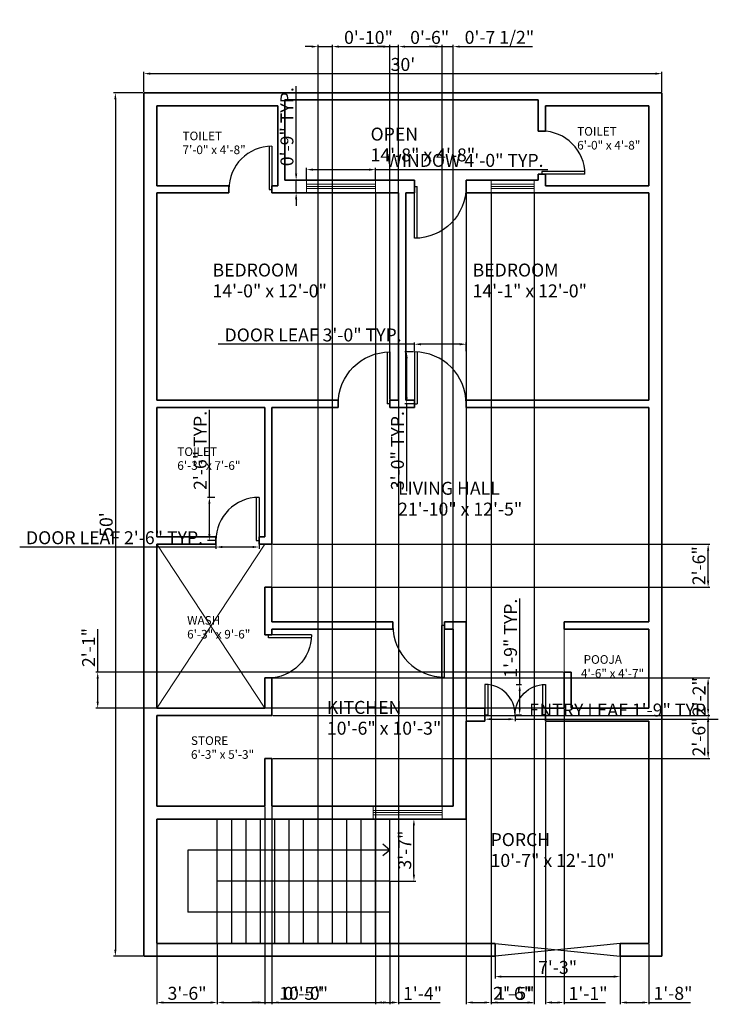
# Model space of a CAD drawing. Units: inches. Extents: x 2391 to 2876, y 1306 to 1990.
import ezdxf

# ---------------------------------------------------------------- set-up
doc = ezdxf.new("R2010")
doc.units = ezdxf.units.IN
for name, color, linetype, lineweight in [('A-ANNO-DIMS', 253, 'Continuous', 18), ('A-AREA-IDEN', 11, 'Continuous', 25), ('A-DOOR', 4, 'Continuous', 25), ('A-FLOR', 11, 'Continuous', 13), ('A-FLOR-STRS', 7, 'Continuous', 25), ('A-GLAZ', 11, 'Continuous', 18), ('A-WALL', 7, 'Continuous', 35), ('A-WALL-OPEN', 11, 'Continuous', 18)]:
    doc.layers.add(name, color=color, linetype=linetype, lineweight=lineweight)
doc.styles.get("Standard").update_dxf_attribs({"font": 'arial.ttf'})
doc.dimstyles.new('ISO-25', dxfattribs={"dimtxt": 9, "dimasz": 4.5, "dimexe": 1.25, "dimexo": 0.625, "dimtad": 1, "dimdec": 0, "dimlunit": 3, "dimtxsty": 'Standard', "dimcen": 2.5, "dimadec": 0, "dimazin": 0, "dimtfac": 1, "dimtdec": 0, "dimtmove": 0, "dimatfit": 3, "dimfxl": 1, "dimarcsym": 0})

# ---------------------------------------------------------------- blocks, each defined once
blk = doc.blocks.new('*D1')
at = {"layer": 'A-ANNO-DIMS', "color": 0, "lineweight": -2, "transparency": 16777216}
for p, q in [((2648.65, 1434.82), (2665.92, 1434.82)), ((2664.67, 1396.12), (2664.67, 1430.32)), ((2648.65, 1391.62), (2665.92, 1391.62))]:
    blk.add_line(p, q, dxfattribs=at)
at = {"layer": 'A-ANNO-DIMS', "color": 0, "transparency": 16777216}
for points in [[(2663.92, 1430.32), (2665.42, 1430.32), (2664.67, 1434.82)], [(2663.92, 1396.12), (2665.42, 1396.12), (2664.67, 1391.62)]]:
    blk.add_solid(points, dxfattribs=at)
at = {"layer": 'Defpoints', "color": 0, "transparency": 16777216}
for p in [(2648.03, 1434.82), (2664.67, 1434.82), (2648.03, 1391.62)]:
    blk.add_point(p, dxfattribs=at)
at = {"layer": 'A-ANNO-DIMS', "color": 0, "transparency": 16777216, "insert": (2659.45, 1413.22), "char_height": 9, "attachment_point": 5, "rotation": 90}
blk.add_mtext('3\'-7"', dxfattribs=at)
blk = doc.blocks.new('*D2')
at = {"layer": 'A-ANNO-DIMS', "color": 0, "lineweight": -2, "transparency": 16777216}
for p, q in [((2721.03, 1347.79), (2721.03, 1324.07)), ((2808.03, 1347.79), (2808.03, 1324.07)), ((2725.53, 1325.32), (2803.53, 1325.32))]:
    blk.add_line(p, q, dxfattribs=at)
at = {"layer": 'A-ANNO-DIMS', "color": 0, "transparency": 16777216}
for points in [[(2725.53, 1326.07), (2725.53, 1324.57), (2721.03, 1325.32)], [(2803.53, 1326.07), (2803.53, 1324.57), (2808.03, 1325.32)]]:
    blk.add_solid(points, dxfattribs=at)
at = {"layer": 'Defpoints', "color": 0, "transparency": 16777216}
for p in [(2721.03, 1348.42), (2808.03, 1348.42), (2808.03, 1325.32)]:
    blk.add_point(p, dxfattribs=at)
at = {"layer": 'A-ANNO-DIMS', "color": 0, "transparency": 16777216, "insert": (2764.53, 1330.54), "char_height": 9, "attachment_point": 5}
blk.add_mtext('7\'-3"', dxfattribs=at)
blk = doc.blocks.new('*D3')
at = {"layer": 'A-ANNO-DIMS', "color": 0, "lineweight": -2, "transparency": 16777216}
for p, q in [((2477.03, 1940.04), (2477.03, 1953.99)), ((2481.53, 1952.74), (2832.53, 1952.74)), ((2837.03, 1940.04), (2837.03, 1953.99))]:
    blk.add_line(p, q, dxfattribs=at)
at = {"layer": 'A-ANNO-DIMS', "color": 0, "transparency": 16777216}
for points in [[(2481.53, 1953.49), (2481.53, 1951.99), (2477.03, 1952.74)], [(2832.53, 1953.49), (2832.53, 1951.99), (2837.03, 1952.74)]]:
    blk.add_solid(points, dxfattribs=at)
at = {"layer": 'Defpoints', "color": 0, "transparency": 16777216}
for p in [(2837.03, 1952.74), (2477.03, 1939.42), (2837.03, 1939.42)]:
    blk.add_point(p, dxfattribs=at)
at = {"layer": 'A-ANNO-DIMS', "color": 0, "transparency": 16777216, "insert": (2657.03, 1957.96), "char_height": 9, "attachment_point": 5}
blk.add_mtext("30'", dxfattribs=at)
blk = doc.blocks.new('*D4')
at = {"layer": 'A-ANNO-DIMS', "color": 0, "lineweight": -2, "transparency": 16777216}
for p, q in [((2476.4, 1939.42), (2455.95, 1939.42)), ((2457.2, 1934.92), (2457.2, 1343.92)), ((2476.4, 1339.42), (2455.95, 1339.42))]:
    blk.add_line(p, q, dxfattribs=at)
at = {"layer": 'A-ANNO-DIMS', "color": 0, "transparency": 16777216}
for points in [[(2456.45, 1934.92), (2457.95, 1934.92), (2457.2, 1939.42)], [(2456.45, 1343.92), (2457.95, 1343.92), (2457.2, 1339.42)]]:
    blk.add_solid(points, dxfattribs=at)
at = {"layer": 'Defpoints', "color": 0, "transparency": 16777216}
for p in [(2477.03, 1939.42), (2457.2, 1339.42), (2477.03, 1339.42)]:
    blk.add_point(p, dxfattribs=at)
at = {"layer": 'A-ANNO-DIMS', "color": 0, "transparency": 16777216, "insert": (2451.98, 1639.42), "char_height": 9, "attachment_point": 5, "rotation": 90}
blk.add_mtext("50'", dxfattribs=at)
blk = doc.blocks.new('DOOR-LEAF-30IN')
for p, q in [((30, 2), (0, 2)), ((0, 2), (0, 0)), ((30, 0), (0, 0))]:
    blk.add_line(p, q)
blk.add_arc((0, 0), 30, 0, 90)
blk = doc.blocks.new('DOOR-LEAF-36IN')
for p, q in [((0, 0), (-2, 0)), ((-2, -36), (-2, 0)), ((0, -36), (0, 0))]:
    blk.add_line(p, q)
blk.add_arc((0, 0), 36, 180, 270)
blk = doc.blocks.new('WIN-48IN')
for p, q in [((0, 0), (48, 0)), ((0, -9), (0, 0)), ((0, -3), (48, -3)), ((0, -4.5), (48, -4.5)), ((0, -6), (48, -6)), ((48, 0), (48, -9)), ((48, -9), (0, -9))]:
    blk.add_line(p, q)
blk = doc.blocks.new('DOOR-LEAF-21IN')
for p, q in [((0, 21), (0, 0)), ((2, 21), (2, 0)), ((0, 0), (2, 0))]:
    blk.add_line(p, q)
blk.add_arc((0, 0), 21, 0, 90)
blk = doc.blocks.new('*D9')
at = {"layer": 'A-ANNO-DIMS', "color": 0, "lineweight": -2, "transparency": 16777216}
for p, q in [((2527.03, 1623.82), (2390.72, 1623.82)), ((2527.03, 1627.69), (2527.03, 1622.57)), ((2552.53, 1623.82), (2531.53, 1623.82)), ((2557.03, 1627.69), (2557.03, 1622.57))]:
    blk.add_line(p, q, dxfattribs=at)
at = {"layer": 'A-ANNO-DIMS', "color": 0, "transparency": 16777216}
for points in [[(2531.53, 1624.57), (2531.53, 1623.07), (2527.03, 1623.82)], [(2552.53, 1624.57), (2552.53, 1623.07), (2557.03, 1623.82)]]:
    blk.add_solid(points, dxfattribs=at)
at = {"layer": 'Defpoints', "color": 0, "transparency": 16777216}
for p in [(2527.03, 1628.32), (2557.03, 1628.32), (2527.03, 1623.82)]:
    blk.add_point(p, dxfattribs=at)
at = {"layer": 'A-ANNO-DIMS', "color": 0, "transparency": 16777216, "insert": (2456.62, 1629.1), "char_height": 9, "attachment_point": 5}
blk.add_mtext('DOOR LEAF 2\'-6" TYP.', dxfattribs=at)
blk = doc.blocks.new('*D10')
at = {"layer": 'A-ANNO-DIMS', "color": 0, "lineweight": -2, "transparency": 16777216}
for p, q in [((2522.53, 1658.32), (2522.53, 1719.08)), ((2526.4, 1658.32), (2521.28, 1658.32)), ((2522.53, 1632.82), (2522.53, 1653.82)), ((2526.4, 1628.32), (2521.28, 1628.32))]:
    blk.add_line(p, q, dxfattribs=at)
at = {"layer": 'A-ANNO-DIMS', "color": 0, "transparency": 16777216}
for points in [[(2521.78, 1653.82), (2523.28, 1653.82), (2522.53, 1658.32)], [(2521.78, 1632.82), (2523.28, 1632.82), (2522.53, 1628.32)]]:
    blk.add_solid(points, dxfattribs=at)
at = {"layer": 'Defpoints', "color": 0, "transparency": 16777216}
for p in [(2522.53, 1658.32), (2527.03, 1658.32), (2527.03, 1628.32)]:
    blk.add_point(p, dxfattribs=at)
at = {"layer": 'A-ANNO-DIMS', "color": 0, "transparency": 16777216, "insert": (2517.31, 1690.95), "char_height": 9, "attachment_point": 5, "rotation": 90}
blk.add_mtext('2\'-6" TYP.', dxfattribs=at)
blk = doc.blocks.new('*D11')
at = {"layer": 'A-ANNO-DIMS', "color": 0, "lineweight": -2, "transparency": 16777216}
for p, q in [((2665.03, 1759.94), (2665.03, 1765.97)), ((2701.03, 1759.94), (2701.03, 1765.97)), ((2665.03, 1764.72), (2528.72, 1764.72)), ((2696.53, 1764.72), (2669.53, 1764.72))]:
    blk.add_line(p, q, dxfattribs=at)
at = {"layer": 'A-ANNO-DIMS', "color": 0, "transparency": 16777216}
for points in [[(2669.53, 1765.47), (2669.53, 1763.97), (2665.03, 1764.72)], [(2696.53, 1765.47), (2696.53, 1763.97), (2701.03, 1764.72)]]:
    blk.add_solid(points, dxfattribs=at)
at = {"layer": 'Defpoints', "color": 0, "transparency": 16777216}
for p in [(2665.03, 1764.72), (2665.03, 1759.32), (2701.03, 1759.32)]:
    blk.add_point(p, dxfattribs=at)
at = {"layer": 'A-ANNO-DIMS', "color": 0, "transparency": 16777216, "insert": (2594.62, 1770), "char_height": 9, "attachment_point": 5}
blk.add_mtext('DOOR LEAF 3\'-0" TYP.', dxfattribs=at)
blk = doc.blocks.new('*D12')
at = {"layer": 'A-ANNO-DIMS', "color": 0, "lineweight": -2, "transparency": 16777216}
for p, q in [((2664.4, 1759.32), (2658.38, 1759.32)), ((2659.63, 1754.82), (2659.63, 1727.82)), ((2664.4, 1723.32), (2658.38, 1723.32)), ((2659.63, 1723.32), (2659.63, 1662.71))]:
    blk.add_line(p, q, dxfattribs=at)
at = {"layer": 'A-ANNO-DIMS', "color": 0, "transparency": 16777216}
for points in [[(2658.88, 1754.82), (2660.38, 1754.82), (2659.63, 1759.32)], [(2658.88, 1727.82), (2660.38, 1727.82), (2659.63, 1723.32)]]:
    blk.add_solid(points, dxfattribs=at)
at = {"layer": 'Defpoints', "color": 0, "transparency": 16777216}
for p in [(2665.03, 1759.32), (2659.63, 1723.32), (2665.03, 1723.32)]:
    blk.add_point(p, dxfattribs=at)
at = {"layer": 'A-ANNO-DIMS', "color": 0, "transparency": 16777216, "insert": (2654.4, 1690.77), "char_height": 9, "attachment_point": 5, "rotation": 90}
blk.add_mtext('3\'-0" TYP.', dxfattribs=at)
blk = doc.blocks.new('*D13')
at = {"layer": 'A-ANNO-DIMS', "color": 0, "lineweight": -2, "transparency": 16777216}
for p, q in [((2714.03, 1506.69), (2714.03, 1502.92)), ((2735.03, 1506.69), (2735.03, 1502.92)), ((2718.53, 1504.17), (2730.53, 1504.17)), ((2735.03, 1504.17), (2876.21, 1504.17))]:
    blk.add_line(p, q, dxfattribs=at)
at = {"layer": 'A-ANNO-DIMS', "color": 0, "transparency": 16777216}
for points in [[(2718.53, 1504.92), (2718.53, 1503.42), (2714.03, 1504.17)], [(2730.53, 1504.92), (2730.53, 1503.42), (2735.03, 1504.17)]]:
    blk.add_solid(points, dxfattribs=at)
at = {"layer": 'Defpoints', "color": 0, "transparency": 16777216}
for p in [(2714.03, 1507.32), (2735.03, 1507.32), (2735.03, 1504.17)]:
    blk.add_point(p, dxfattribs=at)
at = {"layer": 'A-ANNO-DIMS', "color": 0, "transparency": 16777216, "insert": (2807.87, 1509.39), "char_height": 9, "attachment_point": 5}
blk.add_mtext('ENTRY LEAF 1\'-9" TYP.', dxfattribs=at)
blk = doc.blocks.new('*D14')
at = {"layer": 'A-ANNO-DIMS', "color": 0, "lineweight": -2, "transparency": 16777216}
for p, q in [((2738.18, 1528.32), (2738.18, 1588.08)), ((2735.65, 1528.32), (2739.43, 1528.32)), ((2738.18, 1511.82), (2738.18, 1523.82)), ((2735.65, 1507.32), (2739.43, 1507.32))]:
    blk.add_line(p, q, dxfattribs=at)
at = {"layer": 'A-ANNO-DIMS', "color": 0, "transparency": 16777216}
for points in [[(2737.43, 1523.82), (2738.93, 1523.82), (2738.18, 1528.32)], [(2737.43, 1511.82), (2738.93, 1511.82), (2738.18, 1507.32)]]:
    blk.add_solid(points, dxfattribs=at)
at = {"layer": 'Defpoints', "color": 0, "transparency": 16777216}
for p in [(2735.03, 1528.32), (2738.18, 1528.32), (2735.03, 1507.32)]:
    blk.add_point(p, dxfattribs=at)
at = {"layer": 'A-ANNO-DIMS', "color": 0, "transparency": 16777216, "insert": (2732.96, 1560.45), "char_height": 9, "attachment_point": 5, "rotation": 90}
blk.add_mtext('1\'-9" TYP.', dxfattribs=at)
blk = doc.blocks.new('*D15')
at = {"layer": 'A-ANNO-DIMS', "color": 0, "lineweight": -2, "transparency": 16777216}
for p, q in [((2590.03, 1879.44), (2590.03, 1887.27)), ((2594.53, 1886.02), (2633.53, 1886.02)), ((2638.03, 1879.44), (2638.03, 1887.27)), ((2638.03, 1886.02), (2757.67, 1886.02))]:
    blk.add_line(p, q, dxfattribs=at)
at = {"layer": 'A-ANNO-DIMS', "color": 0, "transparency": 16777216}
for points in [[(2594.53, 1886.77), (2594.53, 1885.27), (2590.03, 1886.02)], [(2633.53, 1886.77), (2633.53, 1885.27), (2638.03, 1886.02)]]:
    blk.add_solid(points, dxfattribs=at)
at = {"layer": 'Defpoints', "color": 0, "transparency": 16777216}
for p in [(2638.03, 1886.02), (2590.03, 1878.82), (2638.03, 1878.82)]:
    blk.add_point(p, dxfattribs=at)
at = {"layer": 'A-ANNO-DIMS', "color": 0, "transparency": 16777216, "insert": (2700.1, 1891.3), "char_height": 9, "attachment_point": 5}
blk.add_mtext('WINDOW 4\'-0" TYP.', dxfattribs=at)
blk = doc.blocks.new('*D16')
at = {"layer": 'A-ANNO-DIMS', "color": 0, "lineweight": -2, "transparency": 16777216}
for p, q in [((2582.83, 1883.32), (2582.83, 1943.93)), ((2589.4, 1878.82), (2581.58, 1878.82)), ((2582.83, 1869.82), (2582.83, 1878.82)), ((2589.4, 1869.82), (2581.58, 1869.82)), ((2582.83, 1865.32), (2582.83, 1860.82))]:
    blk.add_line(p, q, dxfattribs=at)
at = {"layer": 'A-ANNO-DIMS', "color": 0, "transparency": 16777216}
for points in [[(2582.08, 1883.32), (2583.58, 1883.32), (2582.83, 1878.82)], [(2582.08, 1865.32), (2583.58, 1865.32), (2582.83, 1869.82)]]:
    blk.add_solid(points, dxfattribs=at)
at = {"layer": 'Defpoints', "color": 0, "transparency": 16777216}
for p in [(2582.83, 1878.82), (2590.03, 1878.82), (2590.03, 1869.82)]:
    blk.add_point(p, dxfattribs=at)
at = {"layer": 'A-ANNO-DIMS', "color": 0, "transparency": 16777216, "insert": (2577.61, 1915.87), "char_height": 9, "attachment_point": 5, "rotation": 90}
blk.add_mtext('0\'-9" TYP.', dxfattribs=at)
blk = doc.blocks.new('*D17')
at = {"layer": 'A-ANNO-DIMS', "color": 0, "lineweight": -2, "transparency": 16777216}
for p, q in [((2444.93, 1536.82), (2444.93, 1566.65)), ((2768.4, 1536.82), (2443.68, 1536.82)), ((2444.93, 1516.32), (2444.93, 1532.32)), ((2768.4, 1511.82), (2443.68, 1511.82))]:
    blk.add_line(p, q, dxfattribs=at)
at = {"layer": 'A-ANNO-DIMS', "color": 0, "transparency": 16777216}
for points in [[(2444.18, 1532.32), (2445.68, 1532.32), (2444.93, 1536.82)], [(2444.18, 1516.32), (2445.68, 1516.32), (2444.93, 1511.82)]]:
    blk.add_solid(points, dxfattribs=at)
at = {"layer": 'Defpoints', "color": 0, "transparency": 16777216}
for p in [(2444.93, 1536.82), (2769.03, 1536.82), (2769.03, 1511.82)]:
    blk.add_point(p, dxfattribs=at)
at = {"layer": 'A-ANNO-DIMS', "color": 0, "transparency": 16777216, "insert": (2439.78, 1553.98), "char_height": 9, "attachment_point": 5, "rotation": 90}
blk.add_mtext('2\'-1"', dxfattribs=at)
blk = doc.blocks.new('*D18')
at = {"layer": 'A-ANNO-DIMS', "color": 0, "lineweight": -2, "transparency": 16777216}
for p, q in [((2528.03, 1347.79), (2528.03, 1306.07)), ((2648.03, 1347.79), (2648.03, 1306.07)), ((2532.53, 1307.32), (2643.53, 1307.32))]:
    blk.add_line(p, q, dxfattribs=at)
at = {"layer": 'A-ANNO-DIMS', "color": 0, "transparency": 16777216}
for points in [[(2532.53, 1308.07), (2532.53, 1306.57), (2528.03, 1307.32)], [(2643.53, 1308.07), (2643.53, 1306.57), (2648.03, 1307.32)]]:
    blk.add_solid(points, dxfattribs=at)
at = {"layer": 'Defpoints', "color": 0, "transparency": 16777216}
for p in [(2528.03, 1348.42), (2648.03, 1348.42), (2648.03, 1307.32)]:
    blk.add_point(p, dxfattribs=at)
at = {"layer": 'A-ANNO-DIMS', "color": 0, "transparency": 16777216, "insert": (2588.03, 1312.54), "char_height": 9, "attachment_point": 5}
blk.add_mtext('10\'-0"', dxfattribs=at)
blk = doc.blocks.new('*D19')
at = {"layer": 'A-ANNO-DIMS', "color": 0, "lineweight": -2, "transparency": 16777216}
for p, q in [((2486.03, 1347.79), (2486.03, 1306.07)), ((2528.03, 1347.79), (2528.03, 1306.07)), ((2490.53, 1307.32), (2523.53, 1307.32))]:
    blk.add_line(p, q, dxfattribs=at)
at = {"layer": 'A-ANNO-DIMS', "color": 0, "transparency": 16777216}
for points in [[(2490.53, 1308.07), (2490.53, 1306.57), (2486.03, 1307.32)], [(2523.53, 1308.07), (2523.53, 1306.57), (2528.03, 1307.32)]]:
    blk.add_solid(points, dxfattribs=at)
at = {"layer": 'Defpoints', "color": 0, "transparency": 16777216}
for p in [(2486.03, 1348.42), (2528.03, 1348.42), (2528.03, 1307.32)]:
    blk.add_point(p, dxfattribs=at)
at = {"layer": 'A-ANNO-DIMS', "color": 0, "transparency": 16777216, "insert": (2507.03, 1312.54), "char_height": 9, "attachment_point": 5}
blk.add_mtext('3\'-6"', dxfattribs=at)
blk = doc.blocks.new('*D20')
at = {"layer": 'A-ANNO-DIMS', "color": 0, "lineweight": -2, "transparency": 16777216}
for p, q in [((2808.03, 1347.79), (2808.03, 1306.07)), ((2828.03, 1347.79), (2828.03, 1306.07)), ((2812.53, 1307.32), (2823.53, 1307.32)), ((2828.03, 1307.32), (2856.86, 1307.32))]:
    blk.add_line(p, q, dxfattribs=at)
at = {"layer": 'A-ANNO-DIMS', "color": 0, "transparency": 16777216}
for points in [[(2812.53, 1308.07), (2812.53, 1306.57), (2808.03, 1307.32)], [(2823.53, 1308.07), (2823.53, 1306.57), (2828.03, 1307.32)]]:
    blk.add_solid(points, dxfattribs=at)
at = {"layer": 'Defpoints', "color": 0, "transparency": 16777216}
for p in [(2808.03, 1348.42), (2828.03, 1348.42), (2828.03, 1307.32)]:
    blk.add_point(p, dxfattribs=at)
at = {"layer": 'A-ANNO-DIMS', "color": 0, "transparency": 16777216, "insert": (2844.69, 1312.54), "char_height": 9, "attachment_point": 5}
blk.add_mtext('1\'-8"', dxfattribs=at)
blk = doc.blocks.new('*D21')
at = {"layer": 'A-ANNO-DIMS', "color": 0, "lineweight": -2, "transparency": 16777216}
for p, q in [((2566.65, 1506.82), (2870.38, 1506.82)), ((2869.13, 1481.32), (2869.13, 1502.32)), ((2566.65, 1476.82), (2870.38, 1476.82))]:
    blk.add_line(p, q, dxfattribs=at)
at = {"layer": 'A-ANNO-DIMS', "color": 0, "transparency": 16777216}
for points in [[(2868.38, 1502.32), (2869.88, 1502.32), (2869.13, 1506.82)], [(2868.38, 1481.32), (2869.88, 1481.32), (2869.13, 1476.82)]]:
    blk.add_solid(points, dxfattribs=at)
at = {"layer": 'Defpoints', "color": 0, "transparency": 16777216}
for p in [(2566.03, 1506.82), (2869.13, 1506.82), (2566.03, 1476.82)]:
    blk.add_point(p, dxfattribs=at)
at = {"layer": 'A-ANNO-DIMS', "color": 0, "transparency": 16777216, "insert": (2863.91, 1491.82), "char_height": 9, "attachment_point": 5, "rotation": 90}
blk.add_mtext('2\'-6"', dxfattribs=at)
blk = doc.blocks.new('*D22')
at = {"layer": 'A-ANNO-DIMS', "color": 0, "lineweight": -2, "transparency": 16777216}
for p, q in [((2566.65, 1625.82), (2870.38, 1625.82)), ((2869.13, 1600.32), (2869.13, 1621.32)), ((2566.65, 1595.82), (2870.38, 1595.82))]:
    blk.add_line(p, q, dxfattribs=at)
at = {"layer": 'A-ANNO-DIMS', "color": 0, "transparency": 16777216}
for points in [[(2868.38, 1621.32), (2869.88, 1621.32), (2869.13, 1625.82)], [(2868.38, 1600.32), (2869.88, 1600.32), (2869.13, 1595.82)]]:
    blk.add_solid(points, dxfattribs=at)
at = {"layer": 'Defpoints', "color": 0, "transparency": 16777216}
for p in [(2566.03, 1625.82), (2869.13, 1625.82), (2566.03, 1595.82)]:
    blk.add_point(p, dxfattribs=at)
at = {"layer": 'A-ANNO-DIMS', "color": 0, "transparency": 16777216, "insert": (2863.91, 1610.82), "char_height": 9, "attachment_point": 5, "rotation": 90}
blk.add_mtext('2\'-6"', dxfattribs=at)
blk = doc.blocks.new('*D23')
at = {"layer": 'A-ANNO-DIMS', "color": 0, "lineweight": -2, "transparency": 16777216}
for p, q in [((2566.65, 1532.82), (2870.38, 1532.82)), ((2869.13, 1511.32), (2869.13, 1528.32)), ((2566.65, 1506.82), (2870.38, 1506.82))]:
    blk.add_line(p, q, dxfattribs=at)
at = {"layer": 'A-ANNO-DIMS', "color": 0, "transparency": 16777216}
for points in [[(2868.38, 1528.32), (2869.88, 1528.32), (2869.13, 1532.82)], [(2868.38, 1511.32), (2869.88, 1511.32), (2869.13, 1506.82)]]:
    blk.add_solid(points, dxfattribs=at)
at = {"layer": 'Defpoints', "color": 0, "transparency": 16777216}
for p in [(2566.03, 1532.82), (2869.13, 1532.82), (2566.03, 1506.82)]:
    blk.add_point(p, dxfattribs=at)
at = {"layer": 'A-ANNO-DIMS', "color": 0, "transparency": 16777216, "insert": (2863.98, 1519.82), "char_height": 9, "attachment_point": 5, "rotation": 90}
blk.add_mtext('2\'-2"', dxfattribs=at)
blk = doc.blocks.new('*D24')
at = {"layer": 'A-ANNO-DIMS', "color": 0, "lineweight": -2, "transparency": 16777216}
for p, q in [((2638.03, 1869.19), (2638.03, 1306.07)), ((2654.03, 1869.19), (2654.03, 1306.07)), ((2642.53, 1307.32), (2649.53, 1307.32)), ((2654.03, 1307.32), (2682.86, 1307.32))]:
    blk.add_line(p, q, dxfattribs=at)
at = {"layer": 'A-ANNO-DIMS', "color": 0, "transparency": 16777216}
for points in [[(2642.53, 1308.07), (2642.53, 1306.57), (2638.03, 1307.32)], [(2649.53, 1308.07), (2649.53, 1306.57), (2654.03, 1307.32)]]:
    blk.add_solid(points, dxfattribs=at)
at = {"layer": 'Defpoints', "color": 0, "transparency": 16777216}
for p in [(2638.03, 1869.82), (2654.03, 1869.82), (2654.03, 1307.32)]:
    blk.add_point(p, dxfattribs=at)
at = {"layer": 'A-ANNO-DIMS', "color": 0, "transparency": 16777216, "insert": (2670.69, 1312.46), "char_height": 9, "attachment_point": 5}
blk.add_mtext('1\'-4"', dxfattribs=at)
blk = doc.blocks.new('*D25')
at = {"layer": 'A-ANNO-DIMS', "color": 0, "lineweight": -2, "transparency": 16777216}
for p, q in [((2701.03, 1869.19), (2701.03, 1306.07)), ((2718.25, 1869.19), (2718.25, 1306.07)), ((2705.53, 1307.32), (2713.75, 1307.32)), ((2718.25, 1307.32), (2747.07, 1307.32))]:
    blk.add_line(p, q, dxfattribs=at)
at = {"layer": 'A-ANNO-DIMS', "color": 0, "transparency": 16777216}
for points in [[(2705.53, 1308.07), (2705.53, 1306.57), (2701.03, 1307.32)], [(2713.75, 1308.07), (2713.75, 1306.57), (2718.25, 1307.32)]]:
    blk.add_solid(points, dxfattribs=at)
at = {"layer": 'Defpoints', "color": 0, "transparency": 16777216}
for p in [(2701.03, 1869.82), (2718.25, 1869.82), (2718.25, 1307.32)]:
    blk.add_point(p, dxfattribs=at)
at = {"layer": 'A-ANNO-DIMS', "color": 0, "transparency": 16777216, "insert": (2734.91, 1312.54), "char_height": 9, "attachment_point": 5}
blk.add_mtext('1\'-5"', dxfattribs=at)
blk = doc.blocks.new('*D26')
at = {"layer": 'A-ANNO-DIMS', "color": 0, "lineweight": -2, "transparency": 16777216}
for p, q in [((2718.25, 1869.19), (2718.25, 1306.07)), ((2748.25, 1869.19), (2748.25, 1306.07)), ((2722.75, 1307.32), (2743.75, 1307.32))]:
    blk.add_line(p, q, dxfattribs=at)
at = {"layer": 'A-ANNO-DIMS', "color": 0, "transparency": 16777216}
for points in [[(2722.75, 1308.07), (2722.75, 1306.57), (2718.25, 1307.32)], [(2743.75, 1308.07), (2743.75, 1306.57), (2748.25, 1307.32)]]:
    blk.add_solid(points, dxfattribs=at)
at = {"layer": 'Defpoints', "color": 0, "transparency": 16777216}
for p in [(2718.25, 1869.82), (2748.25, 1869.82), (2748.25, 1307.32)]:
    blk.add_point(p, dxfattribs=at)
at = {"layer": 'A-ANNO-DIMS', "color": 0, "transparency": 16777216, "insert": (2733.25, 1312.54), "char_height": 9, "attachment_point": 5}
blk.add_mtext('2\'-6"', dxfattribs=at)
blk = doc.blocks.new('*D27')
at = {"layer": 'A-ANNO-DIMS', "color": 0, "lineweight": -2, "transparency": 16777216}
for p, q in [((2643.53, 1971.52), (2639.03, 1971.52)), ((2648.03, 1726.44), (2648.03, 1972.77)), ((2648.03, 1971.52), (2654.03, 1971.52)), ((2654.03, 1726.44), (2654.03, 1972.77)), ((2658.53, 1971.52), (2688.2, 1971.52))]:
    blk.add_line(p, q, dxfattribs=at)
at = {"layer": 'A-ANNO-DIMS', "color": 0, "transparency": 16777216}
for points in [[(2643.53, 1972.27), (2643.53, 1970.77), (2648.03, 1971.52)], [(2658.53, 1972.27), (2658.53, 1970.77), (2654.03, 1971.52)]]:
    blk.add_solid(points, dxfattribs=at)
at = {"layer": 'Defpoints', "color": 0, "transparency": 16777216}
for p in [(2654.03, 1971.52), (2648.03, 1725.82), (2654.03, 1725.82)]:
    blk.add_point(p, dxfattribs=at)
at = {"layer": 'A-ANNO-DIMS', "color": 0, "transparency": 16777216, "insert": (2675.62, 1976.74), "char_height": 9, "attachment_point": 5}
blk.add_mtext('0\'-6"', dxfattribs=at)
blk = doc.blocks.new('*D28')
at = {"layer": 'A-ANNO-DIMS', "color": 0, "lineweight": -2, "transparency": 16777216}
for p, q in [((2769.03, 1511.19), (2769.03, 1306.07)), ((2756.03, 1502.19), (2756.03, 1306.07)), ((2760.53, 1307.32), (2764.53, 1307.32)), ((2769.03, 1307.32), (2797.86, 1307.32))]:
    blk.add_line(p, q, dxfattribs=at)
at = {"layer": 'A-ANNO-DIMS', "color": 0, "transparency": 16777216}
for points in [[(2760.53, 1308.07), (2760.53, 1306.57), (2756.03, 1307.32)], [(2764.53, 1308.07), (2764.53, 1306.57), (2769.03, 1307.32)]]:
    blk.add_solid(points, dxfattribs=at)
at = {"layer": 'Defpoints', "color": 0, "transparency": 16777216}
for p in [(2769.03, 1511.82), (2756.03, 1502.82), (2769.03, 1307.32)]:
    blk.add_point(p, dxfattribs=at)
at = {"layer": 'A-ANNO-DIMS', "color": 0, "transparency": 16777216, "insert": (2785.69, 1312.46), "char_height": 9, "attachment_point": 5}
blk.add_mtext('1\'-1"', dxfattribs=at)
blk = doc.blocks.new('*D29')
at = {"layer": 'A-ANNO-DIMS', "color": 0, "lineweight": -2, "transparency": 16777216}
for p, q in [((2679.81, 1971.52), (2675.31, 1971.52)), ((2684.31, 1444.44), (2684.31, 1972.77)), ((2684.31, 1971.52), (2692.03, 1971.52)), ((2692.03, 1444.44), (2692.03, 1972.77)), ((2696.53, 1971.52), (2747.17, 1971.52))]:
    blk.add_line(p, q, dxfattribs=at)
at = {"layer": 'A-ANNO-DIMS', "color": 0, "transparency": 16777216}
for points in [[(2679.81, 1972.27), (2679.81, 1970.77), (2684.31, 1971.52)], [(2696.53, 1972.27), (2696.53, 1970.77), (2692.03, 1971.52)]]:
    blk.add_solid(points, dxfattribs=at)
at = {"layer": 'Defpoints', "color": 0, "transparency": 16777216}
for p in [(2692.03, 1971.52), (2684.31, 1443.82), (2692.03, 1443.82)]:
    blk.add_point(p, dxfattribs=at)
at = {"layer": 'A-ANNO-DIMS', "color": 0, "transparency": 16777216, "insert": (2724.1, 1976.8), "char_height": 9, "attachment_point": 5}
blk.add_mtext('0\'-7 1/2"', dxfattribs=at)
blk = doc.blocks.new('*D30')
at = {"layer": 'A-ANNO-DIMS', "color": 0, "lineweight": -2, "transparency": 16777216}
for p, q in [((2561.03, 1443.19), (2561.03, 1306.07)), ((2566.03, 1443.19), (2566.03, 1306.07)), ((2556.53, 1307.32), (2552.03, 1307.32)), ((2561.03, 1307.32), (2566.03, 1307.32)), ((2570.53, 1307.32), (2600.2, 1307.32))]:
    blk.add_line(p, q, dxfattribs=at)
at = {"layer": 'A-ANNO-DIMS', "color": 0, "transparency": 16777216}
for points in [[(2556.53, 1308.07), (2556.53, 1306.57), (2561.03, 1307.32)], [(2570.53, 1308.07), (2570.53, 1306.57), (2566.03, 1307.32)]]:
    blk.add_solid(points, dxfattribs=at)
at = {"layer": 'Defpoints', "color": 0, "transparency": 16777216}
for p in [(2561.03, 1443.82), (2566.03, 1443.82), (2566.03, 1307.32)]:
    blk.add_point(p, dxfattribs=at)
at = {"layer": 'A-ANNO-DIMS', "color": 0, "transparency": 16777216, "insert": (2587.62, 1312.54), "char_height": 9, "attachment_point": 5}
blk.add_mtext('0\'-5"', dxfattribs=at)
blk = doc.blocks.new('*D31')
at = {"layer": 'A-ANNO-DIMS', "color": 0, "lineweight": -2, "transparency": 16777216}
for p, q in [((2593.53, 1971.52), (2589.03, 1971.52)), ((2598.03, 1435.44), (2598.03, 1972.77)), ((2598.03, 1971.52), (2608.03, 1971.52)), ((2608.03, 1435.44), (2608.03, 1972.77)), ((2612.53, 1971.52), (2649.19, 1971.52))]:
    blk.add_line(p, q, dxfattribs=at)
at = {"layer": 'A-ANNO-DIMS', "color": 0, "transparency": 16777216}
for points in [[(2593.53, 1972.27), (2593.53, 1970.77), (2598.03, 1971.52)], [(2612.53, 1972.27), (2612.53, 1970.77), (2608.03, 1971.52)]]:
    blk.add_solid(points, dxfattribs=at)
at = {"layer": 'Defpoints', "color": 0, "transparency": 16777216}
for p in [(2608.03, 1971.52), (2598.03, 1434.82), (2608.03, 1434.82)]:
    blk.add_point(p, dxfattribs=at)
at = {"layer": 'A-ANNO-DIMS', "color": 0, "transparency": 16777216, "insert": (2633.11, 1976.74), "char_height": 9, "attachment_point": 5}
blk.add_mtext('0\'-10"', dxfattribs=at)

msp = doc.modelspace()

# ---------------------------------------------------------------- linework, layer by layer
at = {"layer": 'A-DOOR'}
for p, q in [((2753.53, 1882.82), (2751.53, 1882.82)), ((2721.03, 1348.42), (2808.03, 1339.42)), ((2808.03, 1348.42), (2721.03, 1339.42))]:
    msp.add_line(p, q, dxfattribs=at)
at = {"layer": 'A-FLOR'}
for p, q in [((2486.03, 1625.82), (2561.03, 1511.82)), ((2561.03, 1625.82), (2486.03, 1511.82))]:
    msp.add_line(p, q, dxfattribs=at)
at = {"layer": 'A-FLOR-STRS'}
for p, q in [((2528.03, 1348.42), (2528.03, 1434.82)), ((2538.03, 1348.42), (2538.03, 1434.82)), ((2548.03, 1348.42), (2548.03, 1434.82)), ((2558.03, 1348.42), (2558.03, 1434.82)), ((2568.03, 1348.42), (2568.03, 1434.82)), ((2578.03, 1348.42), (2578.03, 1434.82)), ((2588.03, 1348.42), (2588.03, 1434.82)), ((2598.03, 1348.42), (2598.03, 1434.82)), ((2608.03, 1348.42), (2608.03, 1434.82)), ((2618.03, 1348.42), (2618.03, 1434.82)), ((2628.03, 1348.42), (2628.03, 1434.82)), ((2638.03, 1348.42), (2638.03, 1434.82)), ((2648.03, 1348.42), (2648.03, 1434.82)), ((2648.03, 1391.62), (2648.03, 1434.82)), ((2648.03, 1413.22), (2643, 1417.29)), ((2648.03, 1413.22), (2507.48, 1413.22)), ((2507.48, 1413.22), (2507.48, 1370.02)), ((2648.03, 1413.22), (2643, 1409.15)), ((2648.03, 1391.62), (2528.03, 1391.62)), ((2648.03, 1391.62), (2648.03, 1348.42)), ((2648.03, 1370.02), (2507.48, 1370.02))]:
    msp.add_line(p, q, dxfattribs=at)
at = {"layer": 'A-GLAZ'}
for p, q in [((2718.25, 1878.82), (2718.25, 1869.82)), ((2718.25, 1878.82), (2748.25, 1878.82)), ((2748.25, 1875.82), (2718.25, 1875.82)), ((2748.25, 1878.82), (2748.25, 1869.82)), ((2748.25, 1874.32), (2718.25, 1874.32)), ((2748.25, 1872.82), (2718.25, 1872.82)), ((2718.25, 1869.82), (2748.25, 1869.82))]:
    msp.add_line(p, q, dxfattribs=at)
at = {"layer": 'A-WALL'}
for p, q in [((2477.03, 1939.42), (2837.03, 1939.42)), ((2477.03, 1339.42), (2477.03, 1939.42)), ((2837.03, 1939.42), (2837.03, 1339.42)), ((2486.03, 1930.42), (2570.03, 1930.42)), ((2486.03, 1874.82), (2486.03, 1930.42)), ((2570.03, 1874.82), (2570.03, 1930.42)), ((2575.03, 1878.82), (2575.03, 1934.42)), ((2575.03, 1934.42), (2751.03, 1934.42)), ((2751.03, 1934.42), (2751.03, 1912.82)), ((2756.03, 1930.42), (2756.03, 1912.82)), ((2756.03, 1930.42), (2828.03, 1930.42)), ((2828.03, 1930.42), (2828.03, 1874.82)), ((2751.03, 1912.82), (2756.03, 1912.82)), ((2751.03, 1882.82), (2756.03, 1882.82)), ((2751.03, 1882.82), (2751.03, 1878.82)), ((2756.03, 1882.82), (2756.03, 1874.82)), ((2486.03, 1874.82), (2536.03, 1874.82)), ((2536.03, 1869.82), (2536.03, 1874.82)), ((2566.03, 1869.82), (2566.03, 1874.82)), ((2566.03, 1874.82), (2570.03, 1874.82)), ((2575.03, 1878.82), (2665.03, 1878.82)), ((2665.03, 1869.82), (2665.03, 1878.82)), ((2701.03, 1869.82), (2701.03, 1878.82)), ((2701.03, 1878.82), (2751.03, 1878.82)), ((2756.03, 1874.82), (2828.03, 1874.82)), ((2486.03, 1869.82), (2536.03, 1869.82)), ((2486.03, 1725.82), (2486.03, 1869.82)), ((2566.03, 1869.82), (2654.03, 1869.82)), ((2654.03, 1725.82), (2654.03, 1869.82)), ((2659.03, 1725.82), (2659.03, 1869.82)), ((2659.03, 1869.82), (2665.03, 1869.82)), ((2701.03, 1869.82), (2828.03, 1869.82)), ((2828.03, 1869.82), (2828.03, 1725.82)), ((2486.03, 1725.82), (2612.03, 1725.82)), ((2612.03, 1720.82), (2612.03, 1725.82)), ((2648.03, 1720.82), (2648.03, 1725.82)), ((2648.03, 1725.82), (2654.03, 1725.82)), ((2659.03, 1725.82), (2665.03, 1725.82)), ((2665.03, 1720.82), (2665.03, 1725.82)), ((2665.03, 1720.82), (2665.03, 1725.82)), ((2701.03, 1720.82), (2701.03, 1725.82)), ((2701.03, 1725.82), (2828.03, 1725.82)), ((2701.03, 1720.82), (2701.03, 1725.82)), ((2486.03, 1720.82), (2561.03, 1720.82)), ((2486.03, 1630.82), (2486.03, 1720.82)), ((2561.03, 1630.82), (2561.03, 1720.82)), ((2566.03, 1720.82), (2612.03, 1720.82)), ((2566.03, 1625.82), (2566.03, 1720.82)), ((2648.03, 1720.82), (2665.03, 1720.82)), ((2701.03, 1720.82), (2828.03, 1720.82)), ((2828.03, 1720.82), (2828.03, 1571.82)), ((2486.03, 1630.82), (2527.03, 1630.82)), ((2527.03, 1625.82), (2527.03, 1630.82)), ((2557.03, 1625.82), (2557.03, 1630.82)), ((2557.03, 1630.82), (2561.03, 1630.82)), ((2486.03, 1625.82), (2527.03, 1625.82)), ((2486.03, 1511.82), (2486.03, 1625.82)), ((2557.03, 1625.82), (2566.03, 1625.82)), ((2561.03, 1562.82), (2561.03, 1595.82)), ((2561.03, 1595.82), (2566.03, 1595.82)), ((2566.03, 1571.82), (2566.03, 1595.82)), ((2566.03, 1571.82), (2650.03, 1571.82)), ((2566.03, 1566.82), (2650.03, 1566.82)), ((2566.03, 1562.82), (2566.03, 1566.82)), ((2650.03, 1566.82), (2650.03, 1571.82)), ((2686.03, 1566.82), (2686.03, 1571.82)), ((2686.03, 1571.82), (2701.03, 1571.82)), ((2686.03, 1566.82), (2692.03, 1566.82)), ((2692.03, 1443.82), (2692.03, 1566.82)), ((2701.03, 1511.82), (2701.03, 1571.82)), ((2769.03, 1571.82), (2769.03, 1566.82)), ((2769.03, 1571.82), (2828.03, 1571.82)), ((2769.03, 1566.82), (2828.03, 1566.82)), ((2828.03, 1566.82), (2828.03, 1511.82)), ((2561.03, 1562.82), (2566.03, 1562.82)), ((2561.03, 1532.82), (2566.03, 1532.82)), ((2561.03, 1511.82), (2561.03, 1532.82)), ((2566.03, 1506.82), (2566.03, 1532.82)), ((2769.03, 1536.82), (2774.03, 1536.82)), ((2769.03, 1536.82), (2769.03, 1511.82)), ((2774.03, 1536.82), (2774.03, 1511.82)), ((2486.03, 1511.82), (2561.03, 1511.82)), ((2486.03, 1506.82), (2566.03, 1506.82)), ((2486.03, 1443.82), (2486.03, 1506.82)), ((2701.03, 1511.82), (2714.03, 1511.82)), ((2701.03, 1511.82), (2714.03, 1511.82)), ((2714.03, 1511.82), (2714.03, 1502.82)), ((2756.03, 1511.82), (2756.03, 1502.82)), ((2756.03, 1511.82), (2769.03, 1511.82)), ((2756.03, 1511.82), (2769.03, 1511.82)), ((2774.03, 1511.82), (2828.03, 1511.82)), ((2701.03, 1434.82), (2701.03, 1502.82)), ((2701.03, 1502.82), (2714.03, 1502.82)), ((2756.03, 1502.82), (2828.03, 1502.82)), ((2828.03, 1502.82), (2828.03, 1348.42)), ((2561.03, 1443.82), (2561.03, 1476.82)), ((2561.03, 1476.82), (2566.03, 1476.82)), ((2566.03, 1443.82), (2566.03, 1476.82)), ((2486.03, 1443.82), (2561.03, 1443.82)), ((2566.03, 1443.82), (2692.03, 1443.82)), ((2486.03, 1348.42), (2486.03, 1434.82)), ((2486.03, 1434.82), (2701.03, 1434.82)), ((2721.03, 1348.42), (2486.03, 1348.42)), ((2721.03, 1339.42), (2721.03, 1348.42)), ((2828.03, 1348.42), (2808.03, 1348.42)), ((2808.03, 1348.42), (2808.03, 1339.42)), ((2721.03, 1339.42), (2477.03, 1339.42)), ((2837.03, 1339.42), (2808.03, 1339.42))]:
    msp.add_line(p, q, dxfattribs=at)
at = {"layer": 'A-WALL-OPEN'}
for p, q in [((2566.03, 1625.82), (2566.03, 1595.82)), ((2769.03, 1566.82), (2769.03, 1536.82))]:
    msp.add_line(p, q, dxfattribs=at)

# ---------------------------------------------------------------- block references
at = {"layer": 'A-DOOR'}
for name, p in [('DOOR-LEAF-30IN', (2753.53, 1882.82)), ('DOOR-LEAF-36IN', (2686.03, 1569.32)), ('DOOR-LEAF-21IN', (2714.03, 1507.32))]:
    msp.add_blockref(name, p, dxfattribs=at)
for name, p, rotation in [('DOOR-LEAF-30IN', (2566.03, 1872.32), 90.00000000000003), ('DOOR-LEAF-36IN', (2665.03, 1723.32), 180), ('DOOR-LEAF-30IN', (2557.03, 1628.32), 90.00000000000011)]:
    msp.add_blockref(name, p, dxfattribs=dict(at, rotation=rotation))
at = {"layer": 'A-DOOR', "extrusion": (0, 0, -1), "zscale": -1}
for name, p in [('DOOR-LEAF-36IN', (-2665.03, 1874.32)), ('DOOR-LEAF-21IN', (-2756.03, 1507.32))]:
    msp.add_blockref(name, p, dxfattribs=at)
at = {"layer": 'A-DOOR', "extrusion": (0, 0, -1), "zscale": -1, "rotation": 180}
for name, p in [('DOOR-LEAF-36IN', (-2648.03, 1723.32)), ('DOOR-LEAF-30IN', (-2563.53, 1562.82))]:
    msp.add_blockref(name, p, dxfattribs=at)
at = {"layer": 'A-GLAZ'}
for p in [(2590.03, 1878.82), (2636.31, 1443.82)]:
    msp.add_blockref('WIN-48IN', p, dxfattribs=at)

# ---------------------------------------------------------------- texts
at = {"layer": 'A-AREA-IDEN'}
for s, height, p in [('TOILET', 6, (2778.12, 1909.64)), ('TOILET', 6, (2503.86, 1906.45)), ('OPEN', 9, (2634.56, 1906.21)), ('7\'-0" x 4\'-8"', 6, (2503.86, 1896.81)), ('6\'-0" x 4\'-8"', 6, (2778.12, 1900)), ('14\'-8" x 4\'-8"', 9, (2634.56, 1891.76)), ('BEDROOM', 9, (2524.7, 1811.76)), ('BEDROOM', 9, (2705.45, 1811.76)), ('14\'-0" x 12\'-0"', 9, (2524.7, 1797.3)), ('14\'-1" x 12\'-0"', 9, (2705.45, 1797.3)), ('TOILET', 6, (2500.23, 1687.07)), ('6\'-3" x 7\'-6"', 6, (2500.23, 1677.44)), ('LIVING HALL', 9, (2653.65, 1660.11)), ('21\'-10" x 12\'-5"', 9, (2653.65, 1645.65)), ('WASH ', 6, (2507.08, 1569.85)), ('6\'-3" x 9\'-6"', 6, (2507.08, 1560.21)), (' POOJA', 6, (2780.75, 1542.67)), ('4\'-6" x 4\'-7"', 6, (2780.75, 1533.04)), ('KITCHEN', 9, (2604.2, 1507.87)), ('10\'-6" x 10\'-3"', 9, (2604.2, 1493.41)), ('STORE', 6, (2509.75, 1486.29)), ('6\'-3" x 5\'-3"', 6, (2509.75, 1476.65)), ('PORCH', 9, (2717.94, 1416)), ('10\'-7" x 12\'-10"', 9, (2717.94, 1401.55))]:
    msp.add_text(s, height=height, dxfattribs=at).set_placement(p)

# ---------------------------------------------------------------- dimensions: what is measured, and where the dimension line sits
at = {"layer": 'A-ANNO-DIMS'}
for base, p1, p2, override, picture, middle in [((2692.03, 1971.52), (2684.31, 1443.82), (2692.03, 1443.82), {"dimdec": 1, "dimlfac": 1, "dimrnd": 0, "dimzin": 1, "dimdsep": 46, "dimlunit": 4, "dimfrac": 2}, '*D29', (2724.1, 1976.8)), ((2608.03, 1971.52), (2598.03, 1434.82), (2608.03, 1434.82), {"dimdec": 1, "dimlfac": 1, "dimrnd": 0, "dimzin": 1, "dimdsep": 46, "dimlunit": 4, "dimfrac": 2}, '*D31', (2633.11, 1976.74)), ((2654.03, 1971.52), (2648.03, 1725.82), (2654.03, 1725.82), {"dimdec": 1, "dimlfac": 1, "dimrnd": 0, "dimzin": 1, "dimdsep": 46, "dimlunit": 4, "dimfrac": 2}, '*D27', (2675.62, 1976.74)), ((2837.03, 1952.74), (2477.03, 1939.42), (2837.03, 1939.42), {"dimclrd": 0, "dimclre": 0, "dimclrt": 0}, '*D3', (2657.03, 1957.96)), ((2654.03, 1307.32), (2638.03, 1869.82), (2654.03, 1869.82), {"dimdec": 1, "dimlfac": 1, "dimrnd": 0, "dimzin": 1, "dimdsep": 46, "dimlunit": 4, "dimfrac": 2}, '*D24', (2670.69, 1312.46)), ((2718.25, 1307.32), (2701.03, 1869.82), (2718.25, 1869.82), {"dimdec": 1, "dimlfac": 1, "dimrnd": 0, "dimzin": 1, "dimdsep": 46, "dimlunit": 4, "dimfrac": 2}, '*D25', (2734.91, 1312.54)), ((2748.25, 1307.32), (2718.25, 1869.82), (2748.25, 1869.82), {"dimdec": 1, "dimlfac": 1, "dimrnd": 0, "dimzin": 1, "dimdsep": 46, "dimlunit": 4, "dimfrac": 2}, '*D26', (2733.25, 1312.54)), ((2769.03, 1307.32), (2756.03, 1502.82), (2769.03, 1511.82), {"dimdec": 1, "dimlfac": 1, "dimrnd": 0, "dimzin": 1, "dimdsep": 46, "dimlunit": 4, "dimfrac": 2}, '*D28', (2785.69, 1312.46)), ((2566.03, 1307.32), (2561.03, 1443.82), (2566.03, 1443.82), {"dimdec": 1, "dimlfac": 1, "dimrnd": 0, "dimzin": 1, "dimdsep": 46, "dimlunit": 4, "dimfrac": 2}, '*D30', (2587.62, 1312.54)), ((2528.03, 1307.32), (2486.03, 1348.42), (2528.03, 1348.42), {"dimdec": 1, "dimlfac": 1, "dimrnd": 0, "dimzin": 1, "dimdsep": 46, "dimlunit": 4, "dimfrac": 2}, '*D19', (2507.03, 1312.54)), ((2648.03, 1307.32), (2528.03, 1348.42), (2648.03, 1348.42), {"dimdec": 1, "dimlfac": 1, "dimrnd": 0, "dimzin": 1, "dimdsep": 46, "dimlunit": 4, "dimfrac": 2}, '*D18', (2588.03, 1312.54)), ((2808.03, 1325.32), (2721.03, 1348.42), (2808.03, 1348.42), {"dimclrd": 0, "dimclre": 0, "dimclrt": 0}, '*D2', (2764.53, 1330.54)), ((2828.03, 1307.32), (2808.03, 1348.42), (2828.03, 1348.42), {"dimdec": 1, "dimlfac": 1, "dimrnd": 0, "dimzin": 1, "dimdsep": 46, "dimlunit": 4, "dimfrac": 2}, '*D20', (2844.69, 1312.54))]:
    dim = msp.add_linear_dim(base=base, p1=p1, p2=p2, dimstyle='ISO-25', override=override, dxfattribs=at)
    dim.commit()
    dim.dimension.update_dxf_attribs({"geometry": picture, "text_midpoint": middle})
for base, p1, p2, angle, text, picture, middle in [((2582.83, 1878.82), (2590.03, 1869.82), (2590.03, 1878.82), 90, '<> TYP.', '*D16', (2577.61, 1915.87)), ((2665.03, 1764.72), (2701.03, 1759.32), (2665.03, 1759.32), 180, 'DOOR LEAF <> TYP.', '*D11', (2594.62, 1770)), ((2659.63, 1723.32), (2665.03, 1759.32), (2665.03, 1723.32), 270, '<> TYP.', '*D12', (2654.4, 1690.77)), ((2522.53, 1658.32), (2527.03, 1628.32), (2527.03, 1658.32), 90, '<> TYP.', '*D10', (2517.31, 1690.95)), ((2527.03, 1623.82), (2557.03, 1628.32), (2527.03, 1628.32), 180, 'DOOR LEAF <> TYP.', '*D9', (2456.62, 1629.1)), ((2738.18, 1528.32), (2735.03, 1507.32), (2735.03, 1528.32), 90, '<> TYP.', '*D14', (2732.96, 1560.45))]:
    dim = msp.add_linear_dim(base=base, p1=p1, p2=p2, angle=angle, text=text, dimstyle='ISO-25', override={"dimdec": 1, "dimlfac": 1, "dimrnd": 0, "dimzin": 1, "dimdsep": 46, "dimlunit": 4, "dimfrac": 2}, dxfattribs=at)
    dim.commit()
    dim.dimension.update_dxf_attribs({"geometry": picture, "text_midpoint": middle})
for base, p1, p2, override, picture, middle in [((2457.2, 1339.42), (2477.03, 1939.42), (2477.03, 1339.42), {"dimclrd": 0, "dimclre": 0, "dimclrt": 0}, '*D4', (2451.98, 1639.42)), ((2869.13, 1625.82), (2566.03, 1595.82), (2566.03, 1625.82), {"dimdec": 1, "dimlfac": 1, "dimrnd": 0, "dimzin": 1, "dimdsep": 46, "dimlunit": 4, "dimfrac": 2}, '*D22', (2863.91, 1610.82)), ((2444.93, 1536.82), (2769.03, 1511.82), (2769.03, 1536.82), {"dimdec": 1, "dimlfac": 1, "dimrnd": 0, "dimzin": 1, "dimdsep": 46, "dimlunit": 4, "dimfrac": 2}, '*D17', (2439.78, 1553.98)), ((2869.13, 1532.82), (2566.03, 1506.82), (2566.03, 1532.82), {"dimdec": 1, "dimlfac": 1, "dimrnd": 0, "dimzin": 1, "dimdsep": 46, "dimlunit": 4, "dimfrac": 2}, '*D23', (2863.98, 1519.82)), ((2869.13, 1506.82), (2566.03, 1476.82), (2566.03, 1506.82), {"dimdec": 1, "dimlfac": 1, "dimrnd": 0, "dimzin": 1, "dimdsep": 46, "dimlunit": 4, "dimfrac": 2}, '*D21', (2863.91, 1491.82)), ((2664.67, 1434.82), (2648.03, 1391.62), (2648.03, 1434.82), {"dimclrd": 0, "dimclre": 0, "dimclrt": 0}, '*D1', (2659.45, 1413.22))]:
    dim = msp.add_linear_dim(base=base, p1=p1, p2=p2, angle=90, dimstyle='ISO-25', override=override, dxfattribs=at)
    dim.commit()
    dim.dimension.update_dxf_attribs({"geometry": picture, "text_midpoint": middle})
for base, p1, p2, text, picture, middle in [((2638.03, 1886.02), (2590.03, 1878.82), (2638.03, 1878.82), 'WINDOW <> TYP.', '*D15', (2700.1, 1891.3)), ((2735.03, 1504.17), (2714.03, 1507.32), (2735.03, 1507.32), 'ENTRY LEAF <> TYP.', '*D13', (2807.87, 1509.39))]:
    dim = msp.add_linear_dim(base=base, p1=p1, p2=p2, text=text, dimstyle='ISO-25', override={"dimdec": 1, "dimlfac": 1, "dimrnd": 0, "dimzin": 1, "dimdsep": 46, "dimlunit": 4, "dimfrac": 2}, dxfattribs=at)
    dim.commit()
    dim.dimension.update_dxf_attribs({"geometry": picture, "text_midpoint": middle})

doc.saveas('drawing.dxf')
